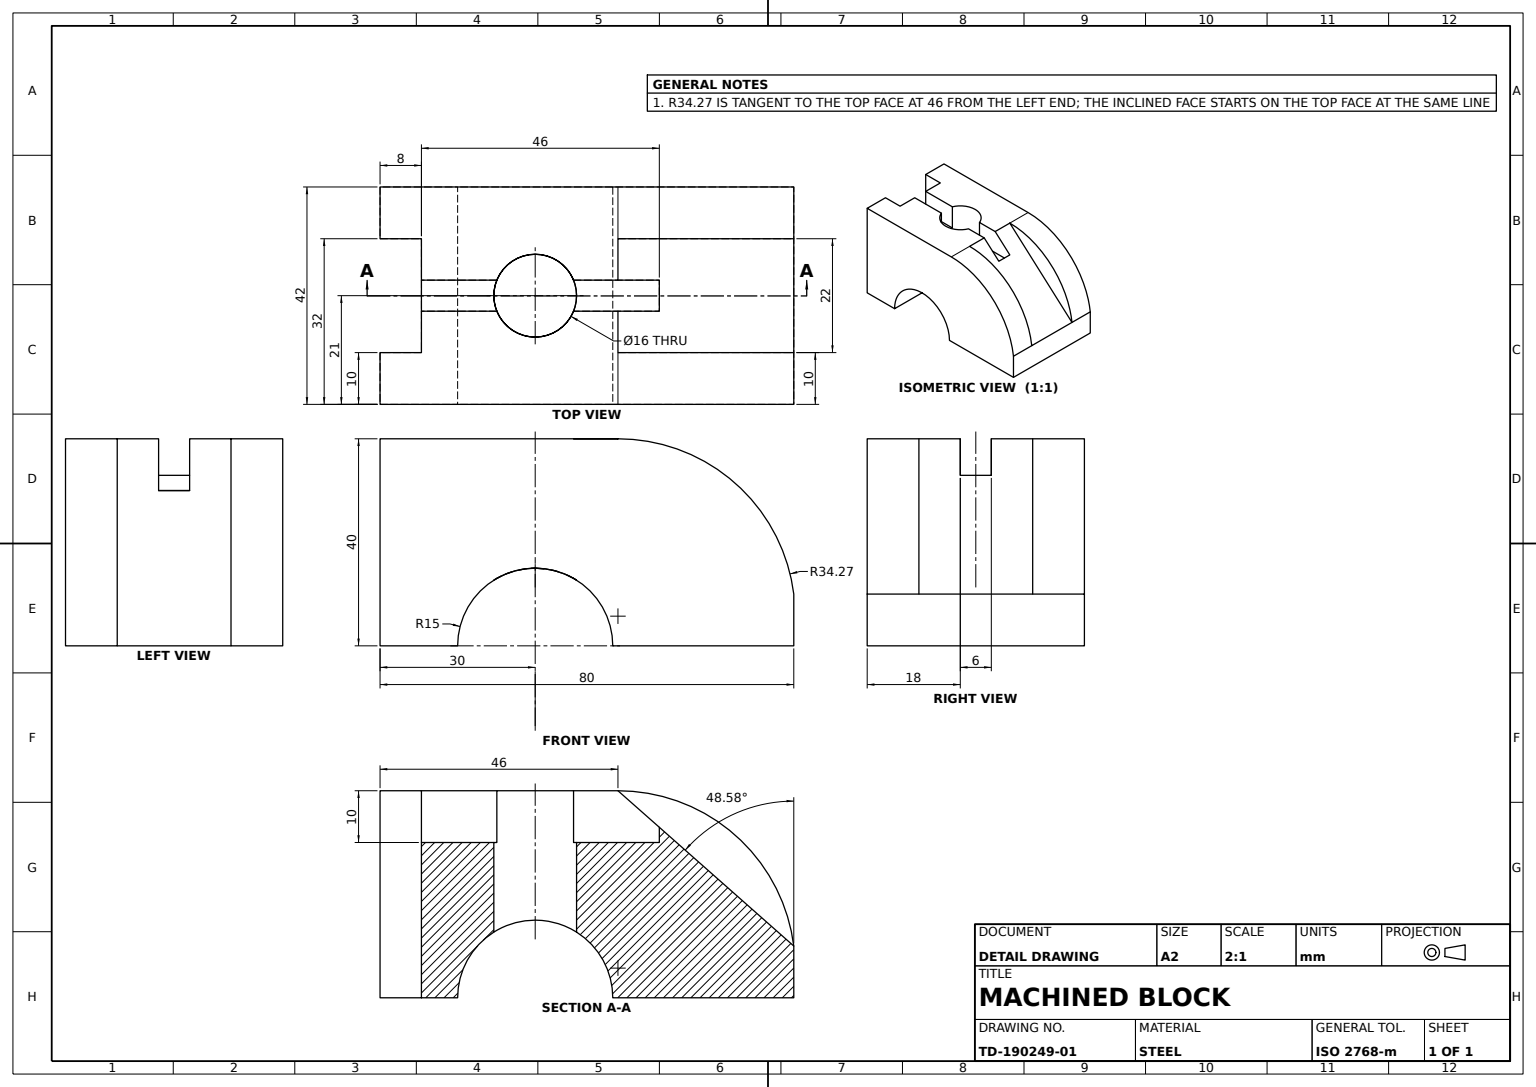
from build123d import *

# Parameters (mm, degrees)
BASE_BLOCK_PROFILE_W        = 80
BASE_BLOCK_PROFILE_H        = 40
BASE_BLOCK_80X40X42_DEPTH   = 42
TOP_SLOT_PROFILE_W          = 34
TOP_SLOT_PROFILE_H          = 30
TOP_SLOT_CUT_10_DEPTH       = 10
GROOVE_CUT_22_DEPTH         = 22
GROOVE_INFILL_BOSS_10_DEPTH = 10
GROOVE_UNDERCUT_10_DEPTH    = 10
ROUNDED_END_CUT_DEPTH       = 42
ARCH_PROFILE_R              = 8
ARCH_CUT_10_DEPTH           = 10
SIDE_SLOT_PROFILE_W         = 22
SIDE_SLOT_PROFILE_H         = 40
SIDE_SLOT_CUT_8_DEPTH       = 8
INCLINED_SLOT_PROFILE_W     = 6
INCLINED_SLOT_PROFILE_H     = 10
INCLINED_SLOT_CUT_46_DEPTH  = 46
BORE_16_PROFILE_R           = 8
BORE_16_CUT_46_DEPTH        = 46


with BuildPart() as part:
    # Base Block Profile → Base Block 80x40x42 (new body)
    with BuildSketch(Plane.XY):
        with Locations((40, 20)):
            Rectangle(BASE_BLOCK_PROFILE_W, BASE_BLOCK_PROFILE_H)
    extrude(amount=-BASE_BLOCK_80X40X42_DEPTH)

    # Top Slot Profile → Top Slot Cut 10 (cut)
    with BuildSketch(Plane.XY):
        with Locations((63, 25)):
            Rectangle(TOP_SLOT_PROFILE_W, TOP_SLOT_PROFILE_H)
    extrude(amount=-TOP_SLOT_CUT_10_DEPTH, mode=Mode.SUBTRACT)

    # Groove Profile → Groove Cut 22 (cut)
    with BuildSketch(Plane.XY.offset(-10)):
        Polygon((46, 40), (80, 10), (80, 40), align=None)
    extrude(amount=-GROOVE_CUT_22_DEPTH, mode=Mode.SUBTRACT)

    # Groove Infill Profile → Groove Infill Boss 10 (add)
    with BuildSketch(Plane.XY):
        with BuildLine():
            Line((46, 40), (46, 10))
            Line((46, 10), (80, 10))
            ThreePointArc((80, 10), (68.671568098, 31.427777177), (46, 40))
        make_face()
    extrude(amount=-GROOVE_INFILL_BOSS_10_DEPTH)

    # Groove Undercut Profile → Groove Undercut 10 (cut)
    with BuildSketch(Plane.XY.offset(-32)):
        with BuildLine():
            Line((46, 40), (80, 40))
            Line((80, 40), (80, 10))
            ThreePointArc((80, 10), (68.671568098, 31.427777177), (46, 40))
        make_face()
    extrude(amount=-GROOVE_UNDERCUT_10_DEPTH, mode=Mode.SUBTRACT)

    # Rounded End Profile → Rounded End Cut (cut)
    with BuildSketch(Plane.XY):
        with BuildLine():
            ThreePointArc((45, 0), (30, 15), (15, 0))
            Line((15, 0), (30, 0))
            Line((30, 0), (45, 0))
        make_face()
    extrude(amount=-ROUNDED_END_CUT_DEPTH, mode=Mode.SUBTRACT)

    # Arch Profile → Arch Cut 10 (cut)
    with BuildSketch(Plane(origin=(0, 40, 0), x_dir=(1, 0, 0), z_dir=(0, 1, 0))):
        with Locations(Location((30, 21, 0), (0, 0, 270))):
            Circle(ARCH_PROFILE_R)
    extrude(amount=-ARCH_CUT_10_DEPTH, mode=Mode.SUBTRACT)

    # Side Slot Profile → Side Slot Cut 8 (cut)
    with BuildSketch(Plane.ZY):
        with Locations((-21, 20)):
            Rectangle(SIDE_SLOT_PROFILE_W, SIDE_SLOT_PROFILE_H)
    extrude(amount=-SIDE_SLOT_CUT_8_DEPTH, mode=Mode.SUBTRACT)

    # Inclined Slot Profile → Inclined Slot Cut 46 (cut)
    with BuildSketch(Plane.ZY.offset(-8)):
        with Locations((-21, 35)):
            Rectangle(INCLINED_SLOT_PROFILE_W, INCLINED_SLOT_PROFILE_H)
    extrude(amount=-INCLINED_SLOT_CUT_46_DEPTH, mode=Mode.SUBTRACT)

    # Bore Ø16 Profile → Bore Ø16 Cut 46 (cut)
    with BuildSketch(Plane(origin=(0, 30, 0), x_dir=(1, 0, 0), z_dir=(0, 1, 0))):
        with Locations(Location((30, 21, 0), (0, 0, 270))):
            Circle(BORE_16_PROFILE_R)
    extrude(amount=-BORE_16_CUT_46_DEPTH, mode=Mode.SUBTRACT)


solid = part.part
